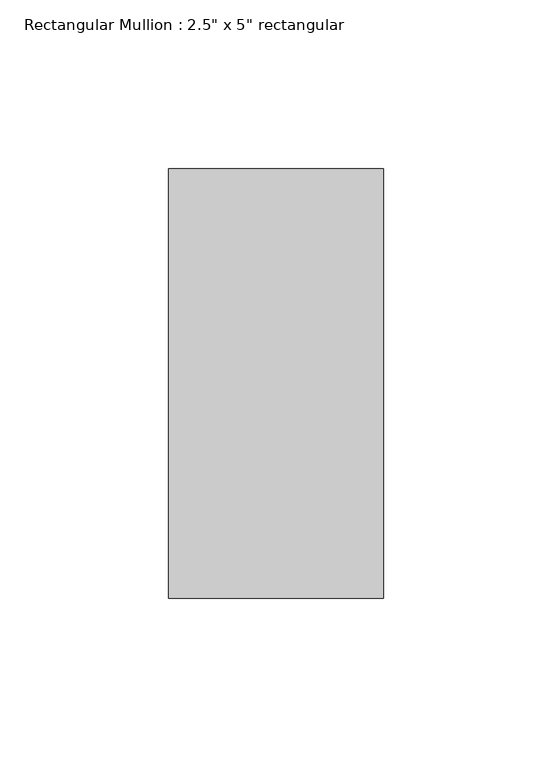
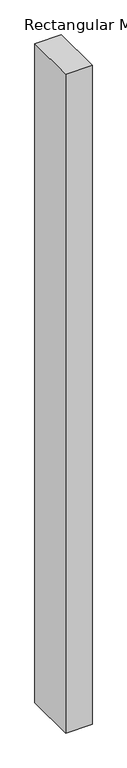
"""IFC4 building model written with IfcOpenShell, lengths in millimetres: member geometry."""

from ifc_helpers import new_model, si_unit, frame, origin, place, context, project, spatial, polyline, outline, extrude, source, transform, mapped, element, save


def member_a448905b(model_context):
    return source(origin(), model_context, "Body", "SweptSolid", [
        extrude(outline(polyline([(0.0, 63.5), (0.0, -63.5), (-63.5, -63.5), (-63.5, 63.5), (0.0, 63.5)])), frame((0.0, 0.0, -1667.45282), z_axis=(0.0, 0.0, 1.0), x_axis=(1.0, 0.0, 0.0)), (0.0, 0.0, 1.0), 1667.45282),
    ])


if __name__ == "__main__":
    model = new_model("IFC4")
    model_context = context("Model", 3, world=origin())
    ifc_project = project(units=[si_unit("LENGTHUNIT", "METRE", prefix="MILLI")], contexts=[model_context])
    site = spatial("IfcSite", under=ifc_project)
    building = spatial("IfcBuilding", under=site)
    placement = place(None, origin())
    member_shape = member_a448905b(model_context)
    element("IfcMember", 1, ObjectType="Rectangular Mullion : 2.5\" x 5\" rectangular", at=placement, inside=building, context=model_context, shape_type="MappedRepresentation", body=[
        mapped(member_shape, transform((0.0, 0.0, 0.0), x_axis=(1.0, 0.0, 0.0), y_axis=(0.0, 1.0, 0.0), z_axis=(0.0, 0.0, 1.0))),
    ])
    save(model, "model.ifc")

# Revit data of these elements
# Type "Rectangular Mullion : 2.5\" x 5\" rectangular"
#   built-in parameter 1007304 = 0.416667 (stored number, unit not read)
#   built-in parameter 1007301 = 0.104167 (stored number, unit not read)
#   built-in parameter 1007300 = 0.104167 (stored number, unit not read)
# Element 1 (IfcMember, "Rectangular Mullion : 2.5\" x 5\" rectangular")
#   Materials on its faces: "Aluminum"
# Materials
#   "Aluminum": class "Metal", colour RGB 247 247 247, transparency 0, Description = "Aluminum 6061", Cost = 0
